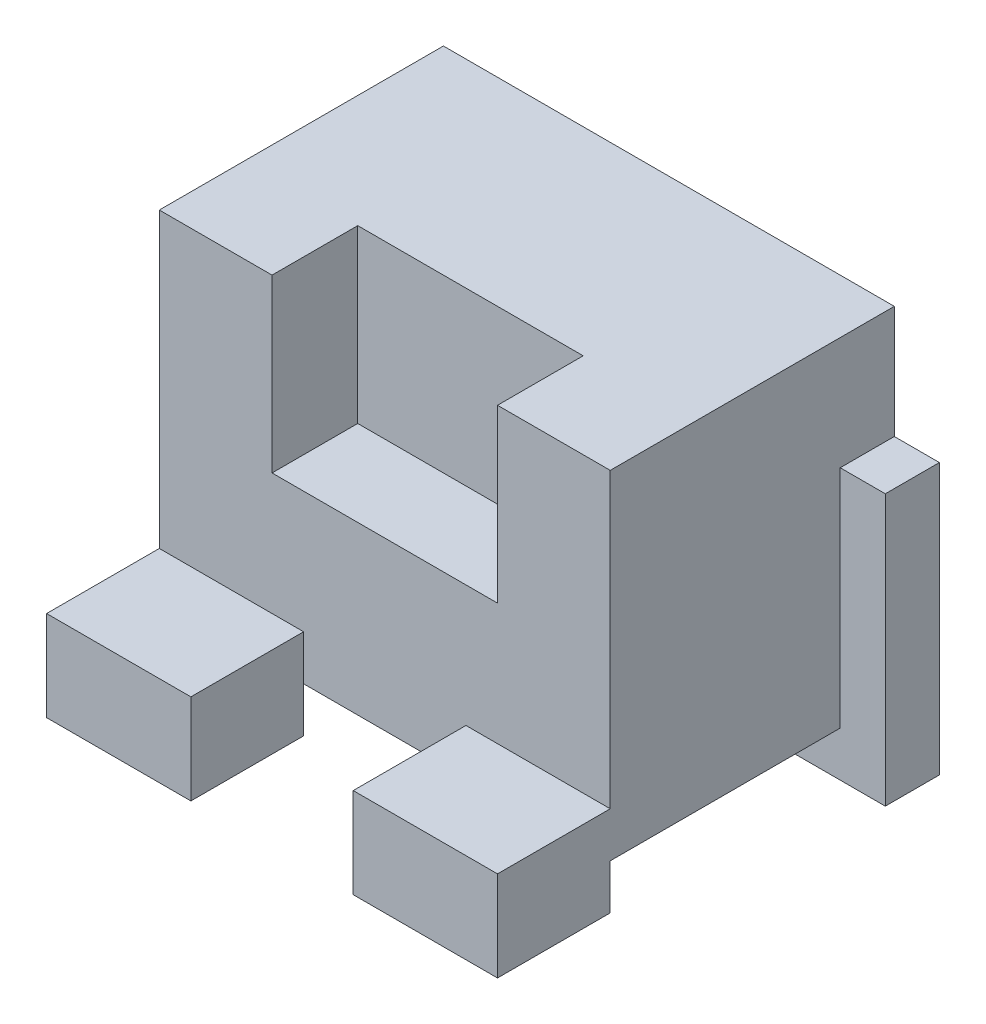
ISO-10303-21;
HEADER;
FILE_DESCRIPTION(('STEP AP214'),'2;1');
FILE_NAME('part.step','',(''),(''),'','','');
FILE_SCHEMA(('AUTOMOTIVE_DESIGN { 1 0 10303 214 1 1 1 1 }'));
ENDSEC;
DATA;
#1=APPLICATION_CONTEXT('core data for automotive mechanical design processes');
#2=APPLICATION_PROTOCOL_DEFINITION('international standard','automotive_design',2000,#1);
#3=PRODUCT_CONTEXT('',#1,'mechanical');
#4=PRODUCT('Part','Part','',(#3));
#5=PRODUCT_RELATED_PRODUCT_CATEGORY('part','',(#4));
#6=PRODUCT_DEFINITION_FORMATION('','',#4);
#7=PRODUCT_DEFINITION_CONTEXT('part definition',#1,'design');
#8=PRODUCT_DEFINITION('design','',#6,#7);
#9=PRODUCT_DEFINITION_SHAPE('','',#8);
#10=(LENGTH_UNIT() NAMED_UNIT(*) SI_UNIT(.MILLI.,.METRE.));
#11=(NAMED_UNIT(*) PLANE_ANGLE_UNIT() SI_UNIT($,.RADIAN.));
#12=(NAMED_UNIT(*) SI_UNIT($,.STERADIAN.) SOLID_ANGLE_UNIT());
#13=UNCERTAINTY_MEASURE_WITH_UNIT(LENGTH_MEASURE(1.E-05),#10,'distance_accuracy_value','');
#14=(GEOMETRIC_REPRESENTATION_CONTEXT(3) GLOBAL_UNCERTAINTY_ASSIGNED_CONTEXT((#13)) GLOBAL_UNIT_ASSIGNED_CONTEXT((#10,
#11,#12)) REPRESENTATION_CONTEXT('',''));
#15=CARTESIAN_POINT('',(0.,0.,0.));
#16=DIRECTION('',(0.,0.,1.));
#17=DIRECTION('',(1.,0.,0.));
#18=AXIS2_PLACEMENT_3D('',#15,#16,#17);
#19=CARTESIAN_POINT('',(100.,75.,-63.));
#20=DIRECTION('',(-1.,0.,0.));
#21=DIRECTION('',(0.,0.,1.));
#22=AXIS2_PLACEMENT_3D('',#19,#20,#21);
#23=PLANE('',#22);
#24=DIRECTION('',(0.,0.,1.));
#25=VECTOR('',#24,1.);
#26=CARTESIAN_POINT('',(100.,50.,-63.));
#27=LINE('',#26,#25);
#28=CARTESIAN_POINT('',(100.,50.,-63.));
#29=VERTEX_POINT('',#28);
#30=CARTESIAN_POINT('',(100.,50.,-51.));
#31=VERTEX_POINT('',#30);
#32=EDGE_CURVE('E231',#29,#31,#27,.T.);
#33=ORIENTED_EDGE('',*,*,#32,.F.);
#34=DIRECTION('',(0.,-1.,0.));
#35=VECTOR('',#34,1.);
#36=CARTESIAN_POINT('',(100.,75.,-63.));
#37=LINE('',#36,#35);
#38=CARTESIAN_POINT('',(100.,75.,-63.));
#39=VERTEX_POINT('',#38);
#40=EDGE_CURVE('E206',#39,#29,#37,.T.);
#41=ORIENTED_EDGE('',*,*,#40,.F.);
#42=DIRECTION('',(0.,0.,-1.));
#43=VECTOR('',#42,1.);
#44=CARTESIAN_POINT('',(100.,75.,-63.));
#45=LINE('',#44,#43);
#46=CARTESIAN_POINT('',(100.,75.,0.));
#47=VERTEX_POINT('',#46);
#48=EDGE_CURVE('E330',#47,#39,#45,.T.);
#49=ORIENTED_EDGE('',*,*,#48,.F.);
#50=DIRECTION('',(0.,-1.,0.));
#51=VECTOR('',#50,1.);
#52=CARTESIAN_POINT('',(100.,75.,0.));
#53=LINE('',#52,#51);
#54=CARTESIAN_POINT('',(100.,9.99999999999999,0.));
#55=VERTEX_POINT('',#54);
#56=EDGE_CURVE('E351',#47,#55,#53,.T.);
#57=ORIENTED_EDGE('',*,*,#56,.T.);
#58=DIRECTION('',(0.,0.,1.));
#59=VECTOR('',#58,1.);
#60=CARTESIAN_POINT('',(100.,10.,0.));
#61=LINE('',#60,#59);
#62=CARTESIAN_POINT('',(100.,10.,25.));
#63=VERTEX_POINT('',#62);
#64=EDGE_CURVE('E250',#55,#63,#61,.T.);
#65=ORIENTED_EDGE('',*,*,#64,.T.);
#66=DIRECTION('',(0.,1.,0.));
#67=VECTOR('',#66,1.);
#68=CARTESIAN_POINT('',(100.,-10.,25.));
#69=LINE('',#68,#67);
#70=CARTESIAN_POINT('',(100.,-10.,25.));
#71=VERTEX_POINT('',#70);
#72=EDGE_CURVE('E256',#71,#63,#69,.T.);
#73=ORIENTED_EDGE('',*,*,#72,.F.);
#74=DIRECTION('',(0.,0.,1.));
#75=VECTOR('',#74,1.);
#76=CARTESIAN_POINT('',(100.,-10.,0.));
#77=LINE('',#76,#75);
#78=CARTESIAN_POINT('',(100.,-10.,0.));
#79=VERTEX_POINT('',#78);
#80=EDGE_CURVE('E239',#79,#71,#77,.T.);
#81=ORIENTED_EDGE('',*,*,#80,.F.);
#82=DIRECTION('',(0.,1.,0.));
#83=VECTOR('',#82,1.);
#84=CARTESIAN_POINT('',(100.,-10.,0.));
#85=LINE('',#84,#83);
#86=CARTESIAN_POINT('',(100.,0.,0.));
#87=VERTEX_POINT('',#86);
#88=EDGE_CURVE('E261',#79,#87,#85,.T.);
#89=ORIENTED_EDGE('',*,*,#88,.T.);
#90=DIRECTION('',(0.,0.,-1.));
#91=VECTOR('',#90,1.);
#92=CARTESIAN_POINT('',(100.,0.,-63.));
#93=LINE('',#92,#91);
#94=CARTESIAN_POINT('',(100.,0.,-51.));
#95=VERTEX_POINT('',#94);
#96=EDGE_CURVE('E337',#87,#95,#93,.T.);
#97=ORIENTED_EDGE('',*,*,#96,.T.);
#98=DIRECTION('',(0.,-1.,0.));
#99=VECTOR('',#98,1.);
#100=CARTESIAN_POINT('',(100.,75.,-51.));
#101=LINE('',#100,#99);
#102=EDGE_CURVE('E207',#31,#95,#101,.T.);
#103=ORIENTED_EDGE('',*,*,#102,.F.);
#104=EDGE_LOOP('',(#33,#41,#49,#57,#65,#73,#81,#89,#97,#103));
#105=FACE_BOUND('',#104,.T.);
#106=ADVANCED_FACE('F39',(#105),#23,.F.);
#107=CARTESIAN_POINT('',(0.,0.,0.));
#108=DIRECTION('',(0.,-1.,0.));
#109=DIRECTION('',(0.,0.,-1.));
#110=AXIS2_PLACEMENT_3D('',#107,#108,#109);
#111=PLANE('',#110);
#112=DIRECTION('',(0.,0.,1.));
#113=VECTOR('',#112,1.);
#114=CARTESIAN_POINT('',(90.,0.,0.));
#115=LINE('',#114,#113);
#116=CARTESIAN_POINT('',(90.,0.,-63.));
#117=VERTEX_POINT('',#116);
#118=CARTESIAN_POINT('',(90.,0.,-51.));
#119=VERTEX_POINT('',#118);
#120=EDGE_CURVE('E50',#117,#119,#115,.T.);
#121=ORIENTED_EDGE('',*,*,#120,.T.);
#122=DIRECTION('',(1.,0.,0.));
#123=VECTOR('',#122,1.);
#124=CARTESIAN_POINT('',(0.,0.,-51.));
#125=LINE('',#124,#123);
#126=EDGE_CURVE('E11',#119,#95,#125,.T.);
#127=ORIENTED_EDGE('',*,*,#126,.T.);
#128=ORIENTED_EDGE('',*,*,#96,.F.);
#129=DIRECTION('',(1.,0.,0.));
#130=VECTOR('',#129,1.);
#131=CARTESIAN_POINT('',(100.,0.,0.));
#132=LINE('',#131,#130);
#133=CARTESIAN_POINT('',(68.,0.,0.));
#134=VERTEX_POINT('',#133);
#135=EDGE_CURVE('E318',#134,#87,#132,.T.);
#136=ORIENTED_EDGE('',*,*,#135,.F.);
#137=CARTESIAN_POINT('',(32.,0.,0.));
#138=VERTEX_POINT('',#137);
#139=EDGE_CURVE('E338',#138,#134,#132,.T.);
#140=ORIENTED_EDGE('',*,*,#139,.F.);
#141=CARTESIAN_POINT('',(0.,0.,0.));
#142=VERTEX_POINT('',#141);
#143=EDGE_CURVE('E333',#142,#138,#132,.T.);
#144=ORIENTED_EDGE('',*,*,#143,.F.);
#145=DIRECTION('',(0.,0.,1.));
#146=VECTOR('',#145,1.);
#147=CARTESIAN_POINT('',(0.,0.,0.));
#148=LINE('',#147,#146);
#149=CARTESIAN_POINT('',(0.,0.,-63.));
#150=VERTEX_POINT('',#149);
#151=EDGE_CURVE('E344',#150,#142,#148,.T.);
#152=ORIENTED_EDGE('',*,*,#151,.F.);
#153=DIRECTION('',(-1.,0.,0.));
#154=VECTOR('',#153,1.);
#155=CARTESIAN_POINT('',(0.,0.,-63.));
#156=LINE('',#155,#154);
#157=EDGE_CURVE('E345',#117,#150,#156,.T.);
#158=ORIENTED_EDGE('',*,*,#157,.F.);
#159=EDGE_LOOP('',(#121,#127,#128,#136,#140,#144,#152,#158));
#160=FACE_BOUND('',#159,.T.);
#161=ADVANCED_FACE('F383',(#160),#111,.T.);
#162=CARTESIAN_POINT('',(100.,75.,0.));
#163=DIRECTION('',(0.,0.,-1.));
#164=DIRECTION('',(-1.,0.,0.));
#165=AXIS2_PLACEMENT_3D('',#162,#163,#164);
#166=PLANE('',#165);
#167=DIRECTION('',(0.,1.,0.));
#168=VECTOR('',#167,1.);
#169=CARTESIAN_POINT('',(68.,-10.,0.));
#170=LINE('',#169,#168);
#171=CARTESIAN_POINT('',(68.,9.99999999999999,0.));
#172=VERTEX_POINT('',#171);
#173=EDGE_CURVE('E65',#134,#172,#170,.T.);
#174=ORIENTED_EDGE('',*,*,#173,.T.);
#175=DIRECTION('',(1.,0.,0.));
#176=VECTOR('',#175,1.);
#177=CARTESIAN_POINT('',(68.,10.,0.));
#178=LINE('',#177,#176);
#179=EDGE_CURVE('E232',#172,#55,#178,.T.);
#180=ORIENTED_EDGE('',*,*,#179,.T.);
#181=ORIENTED_EDGE('',*,*,#56,.F.);
#182=DIRECTION('',(1.,0.,0.));
#183=VECTOR('',#182,1.);
#184=CARTESIAN_POINT('',(100.,75.,0.));
#185=LINE('',#184,#183);
#186=CARTESIAN_POINT('',(75.,75.,0.));
#187=VERTEX_POINT('',#186);
#188=EDGE_CURVE('E327',#187,#47,#185,.T.);
#189=ORIENTED_EDGE('',*,*,#188,.F.);
#190=DIRECTION('',(0.,1.,0.));
#191=VECTOR('',#190,1.);
#192=CARTESIAN_POINT('',(75.,37.,0.));
#193=LINE('',#192,#191);
#194=CARTESIAN_POINT('',(75.,37.,0.));
#195=VERTEX_POINT('',#194);
#196=EDGE_CURVE('E299',#195,#187,#193,.T.);
#197=ORIENTED_EDGE('',*,*,#196,.F.);
#198=DIRECTION('',(1.,0.,0.));
#199=VECTOR('',#198,1.);
#200=CARTESIAN_POINT('',(25.,37.,0.));
#201=LINE('',#200,#199);
#202=CARTESIAN_POINT('',(25.,37.,0.));
#203=VERTEX_POINT('',#202);
#204=EDGE_CURVE('E313',#203,#195,#201,.T.);
#205=ORIENTED_EDGE('',*,*,#204,.F.);
#206=DIRECTION('',(0.,-1.,0.));
#207=VECTOR('',#206,1.);
#208=CARTESIAN_POINT('',(25.,75.,0.));
#209=LINE('',#208,#207);
#210=CARTESIAN_POINT('',(25.,75.,0.));
#211=VERTEX_POINT('',#210);
#212=EDGE_CURVE('E294',#211,#203,#209,.T.);
#213=ORIENTED_EDGE('',*,*,#212,.F.);
#214=CARTESIAN_POINT('',(0.,75.,0.));
#215=VERTEX_POINT('',#214);
#216=EDGE_CURVE('E322',#215,#211,#185,.T.);
#217=ORIENTED_EDGE('',*,*,#216,.F.);
#218=DIRECTION('',(0.,-1.,0.));
#219=VECTOR('',#218,1.);
#220=CARTESIAN_POINT('',(0.,75.,0.));
#221=LINE('',#220,#219);
#222=CARTESIAN_POINT('',(0.,9.99999999999999,0.));
#223=VERTEX_POINT('',#222);
#224=EDGE_CURVE('E331',#215,#223,#221,.T.);
#225=ORIENTED_EDGE('',*,*,#224,.T.);
#226=DIRECTION('',(1.,0.,0.));
#227=VECTOR('',#226,1.);
#228=CARTESIAN_POINT('',(32.,10.,0.));
#229=LINE('',#228,#227);
#230=CARTESIAN_POINT('',(32.,10.,0.));
#231=VERTEX_POINT('',#230);
#232=EDGE_CURVE('E262',#223,#231,#229,.T.);
#233=ORIENTED_EDGE('',*,*,#232,.T.);
#234=DIRECTION('',(0.,1.,0.));
#235=VECTOR('',#234,1.);
#236=CARTESIAN_POINT('',(32.,-10.,0.));
#237=LINE('',#236,#235);
#238=EDGE_CURVE('E293',#138,#231,#237,.T.);
#239=ORIENTED_EDGE('',*,*,#238,.F.);
#240=ORIENTED_EDGE('',*,*,#139,.T.);
#241=EDGE_LOOP('',(#174,#180,#181,#189,#197,#205,#213,#217,#225,#233,#239,#240));
#242=FACE_BOUND('',#241,.T.);
#243=ADVANCED_FACE('F41',(#242),#166,.F.);
#244=CARTESIAN_POINT('',(0.,75.,-63.));
#245=DIRECTION('',(0.,0.,1.));
#246=DIRECTION('',(1.,0.,0.));
#247=AXIS2_PLACEMENT_3D('',#244,#245,#246);
#248=PLANE('',#247);
#249=ORIENTED_EDGE('',*,*,#40,.T.);
#250=DIRECTION('',(-1.,0.,0.));
#251=VECTOR('',#250,1.);
#252=CARTESIAN_POINT('',(110.,50.,-63.));
#253=LINE('',#252,#251);
#254=CARTESIAN_POINT('',(110.,50.,-63.));
#255=VERTEX_POINT('',#254);
#256=EDGE_CURVE('E205',#255,#29,#253,.T.);
#257=ORIENTED_EDGE('',*,*,#256,.F.);
#258=DIRECTION('',(0.,1.,0.));
#259=VECTOR('',#258,1.);
#260=CARTESIAN_POINT('',(110.,-9.99999999999999,-63.));
#261=LINE('',#260,#259);
#262=CARTESIAN_POINT('',(110.,-9.99999999999999,-63.));
#263=VERTEX_POINT('',#262);
#264=EDGE_CURVE('E187',#263,#255,#261,.T.);
#265=ORIENTED_EDGE('',*,*,#264,.F.);
#266=DIRECTION('',(-1.,0.,0.));
#267=VECTOR('',#266,1.);
#268=CARTESIAN_POINT('',(110.,-9.99999999999999,-63.));
#269=LINE('',#268,#267);
#270=CARTESIAN_POINT('',(90.,-9.99999999999999,-63.));
#271=VERTEX_POINT('',#270);
#272=EDGE_CURVE('E219',#263,#271,#269,.T.);
#273=ORIENTED_EDGE('',*,*,#272,.T.);
#274=DIRECTION('',(0.,1.,0.));
#275=VECTOR('',#274,1.);
#276=CARTESIAN_POINT('',(90.,0.,-63.));
#277=LINE('',#276,#275);
#278=EDGE_CURVE('E222',#271,#117,#277,.T.);
#279=ORIENTED_EDGE('',*,*,#278,.T.);
#280=ORIENTED_EDGE('',*,*,#157,.T.);
#281=DIRECTION('',(0.,-1.,0.));
#282=VECTOR('',#281,1.);
#283=CARTESIAN_POINT('',(0.,75.,-63.));
#284=LINE('',#283,#282);
#285=CARTESIAN_POINT('',(0.,75.,-63.));
#286=VERTEX_POINT('',#285);
#287=EDGE_CURVE('E350',#286,#150,#284,.T.);
#288=ORIENTED_EDGE('',*,*,#287,.F.);
#289=DIRECTION('',(-1.,0.,0.));
#290=VECTOR('',#289,1.);
#291=CARTESIAN_POINT('',(0.,75.,-63.));
#292=LINE('',#291,#290);
#293=EDGE_CURVE('E329',#39,#286,#292,.T.);
#294=ORIENTED_EDGE('',*,*,#293,.F.);
#295=EDGE_LOOP('',(#249,#257,#265,#273,#279,#280,#288,#294));
#296=FACE_BOUND('',#295,.T.);
#297=ADVANCED_FACE('F201',(#296),#248,.F.);
#298=CARTESIAN_POINT('',(0.,75.,0.));
#299=DIRECTION('',(1.,0.,0.));
#300=DIRECTION('',(0.,0.,-1.));
#301=AXIS2_PLACEMENT_3D('',#298,#299,#300);
#302=PLANE('',#301);
#303=ORIENTED_EDGE('',*,*,#151,.T.);
#304=DIRECTION('',(0.,1.,0.));
#305=VECTOR('',#304,1.);
#306=CARTESIAN_POINT('',(0.,-10.,0.));
#307=LINE('',#306,#305);
#308=CARTESIAN_POINT('',(0.,-10.,0.));
#309=VERTEX_POINT('',#308);
#310=EDGE_CURVE('E274',#309,#142,#307,.T.);
#311=ORIENTED_EDGE('',*,*,#310,.F.);
#312=DIRECTION('',(0.,0.,-1.));
#313=VECTOR('',#312,1.);
#314=CARTESIAN_POINT('',(0.,-10.,0.));
#315=LINE('',#314,#313);
#316=CARTESIAN_POINT('',(0.,-10.,25.));
#317=VERTEX_POINT('',#316);
#318=EDGE_CURVE('E272',#317,#309,#315,.T.);
#319=ORIENTED_EDGE('',*,*,#318,.F.);
#320=DIRECTION('',(0.,1.,0.));
#321=VECTOR('',#320,1.);
#322=CARTESIAN_POINT('',(0.,-10.,25.));
#323=LINE('',#322,#321);
#324=CARTESIAN_POINT('',(0.,10.,25.));
#325=VERTEX_POINT('',#324);
#326=EDGE_CURVE('E284',#317,#325,#323,.T.);
#327=ORIENTED_EDGE('',*,*,#326,.T.);
#328=DIRECTION('',(0.,0.,-1.));
#329=VECTOR('',#328,1.);
#330=CARTESIAN_POINT('',(0.,10.,0.));
#331=LINE('',#330,#329);
#332=EDGE_CURVE('E267',#325,#223,#331,.T.);
#333=ORIENTED_EDGE('',*,*,#332,.T.);
#334=ORIENTED_EDGE('',*,*,#224,.F.);
#335=DIRECTION('',(0.,0.,1.));
#336=VECTOR('',#335,1.);
#337=CARTESIAN_POINT('',(0.,75.,0.));
#338=LINE('',#337,#336);
#339=EDGE_CURVE('E335',#286,#215,#338,.T.);
#340=ORIENTED_EDGE('',*,*,#339,.F.);
#341=ORIENTED_EDGE('',*,*,#287,.T.);
#342=EDGE_LOOP('',(#303,#311,#319,#327,#333,#334,#340,#341));
#343=FACE_BOUND('',#342,.T.);
#344=ADVANCED_FACE('F372',(#343),#302,.F.);
#345=CARTESIAN_POINT('',(0.,75.,0.));
#346=DIRECTION('',(0.,-1.,0.));
#347=DIRECTION('',(0.,0.,-1.));
#348=AXIS2_PLACEMENT_3D('',#345,#346,#347);
#349=PLANE('',#348);
#350=DIRECTION('',(-1.,0.,0.));
#351=VECTOR('',#350,1.);
#352=CARTESIAN_POINT('',(75.,75.,-19.));
#353=LINE('',#352,#351);
#354=CARTESIAN_POINT('',(75.,75.,-19.));
#355=VERTEX_POINT('',#354);
#356=CARTESIAN_POINT('',(25.,75.,-19.));
#357=VERTEX_POINT('',#356);
#358=EDGE_CURVE('E296',#355,#357,#353,.T.);
#359=ORIENTED_EDGE('',*,*,#358,.F.);
#360=DIRECTION('',(0.,0.,1.));
#361=VECTOR('',#360,1.);
#362=CARTESIAN_POINT('',(75.,75.,-19.));
#363=LINE('',#362,#361);
#364=EDGE_CURVE('E312',#355,#187,#363,.T.);
#365=ORIENTED_EDGE('',*,*,#364,.T.);
#366=ORIENTED_EDGE('',*,*,#188,.T.);
#367=ORIENTED_EDGE('',*,*,#48,.T.);
#368=ORIENTED_EDGE('',*,*,#293,.T.);
#369=ORIENTED_EDGE('',*,*,#339,.T.);
#370=ORIENTED_EDGE('',*,*,#216,.T.);
#371=DIRECTION('',(0.,0.,1.));
#372=VECTOR('',#371,1.);
#373=CARTESIAN_POINT('',(25.,75.,-19.));
#374=LINE('',#373,#372);
#375=EDGE_CURVE('E306',#357,#211,#374,.T.);
#376=ORIENTED_EDGE('',*,*,#375,.F.);
#377=EDGE_LOOP('',(#359,#365,#366,#367,#368,#369,#370,#376));
#378=FACE_BOUND('',#377,.T.);
#379=ADVANCED_FACE('F415',(#378),#349,.F.);
#380=CARTESIAN_POINT('',(75.,37.,-19.));
#381=DIRECTION('',(1.,0.,0.));
#382=DIRECTION('',(0.,0.,-1.));
#383=AXIS2_PLACEMENT_3D('',#380,#381,#382);
#384=PLANE('',#383);
#385=ORIENTED_EDGE('',*,*,#196,.T.);
#386=ORIENTED_EDGE('',*,*,#364,.F.);
#387=DIRECTION('',(0.,1.,0.));
#388=VECTOR('',#387,1.);
#389=CARTESIAN_POINT('',(75.,37.,-19.));
#390=LINE('',#389,#388);
#391=CARTESIAN_POINT('',(75.,37.,-19.));
#392=VERTEX_POINT('',#391);
#393=EDGE_CURVE('E308',#392,#355,#390,.T.);
#394=ORIENTED_EDGE('',*,*,#393,.F.);
#395=DIRECTION('',(0.,0.,1.));
#396=VECTOR('',#395,1.);
#397=CARTESIAN_POINT('',(75.,37.,-19.));
#398=LINE('',#397,#396);
#399=EDGE_CURVE('E317',#392,#195,#398,.T.);
#400=ORIENTED_EDGE('',*,*,#399,.T.);
#401=EDGE_LOOP('',(#385,#386,#394,#400));
#402=FACE_BOUND('',#401,.T.);
#403=ADVANCED_FACE('F420',(#402),#384,.F.);
#404=CARTESIAN_POINT('',(25.,37.,-19.));
#405=DIRECTION('',(0.,-1.,0.));
#406=DIRECTION('',(0.,0.,-1.));
#407=AXIS2_PLACEMENT_3D('',#404,#405,#406);
#408=PLANE('',#407);
#409=ORIENTED_EDGE('',*,*,#204,.T.);
#410=ORIENTED_EDGE('',*,*,#399,.F.);
#411=DIRECTION('',(1.,0.,0.));
#412=VECTOR('',#411,1.);
#413=CARTESIAN_POINT('',(25.,37.,-19.));
#414=LINE('',#413,#412);
#415=CARTESIAN_POINT('',(25.,37.,-19.));
#416=VERTEX_POINT('',#415);
#417=EDGE_CURVE('E301',#416,#392,#414,.T.);
#418=ORIENTED_EDGE('',*,*,#417,.F.);
#419=DIRECTION('',(0.,0.,1.));
#420=VECTOR('',#419,1.);
#421=CARTESIAN_POINT('',(25.,37.,-19.));
#422=LINE('',#421,#420);
#423=EDGE_CURVE('E321',#416,#203,#422,.T.);
#424=ORIENTED_EDGE('',*,*,#423,.T.);
#425=EDGE_LOOP('',(#409,#410,#418,#424));
#426=FACE_BOUND('',#425,.T.);
#427=ADVANCED_FACE('F421',(#426),#408,.F.);
#428=CARTESIAN_POINT('',(25.,75.,-19.));
#429=DIRECTION('',(-1.,0.,0.));
#430=DIRECTION('',(0.,0.,1.));
#431=AXIS2_PLACEMENT_3D('',#428,#429,#430);
#432=PLANE('',#431);
#433=ORIENTED_EDGE('',*,*,#212,.T.);
#434=ORIENTED_EDGE('',*,*,#423,.F.);
#435=DIRECTION('',(0.,-1.,0.));
#436=VECTOR('',#435,1.);
#437=CARTESIAN_POINT('',(25.,75.,-19.));
#438=LINE('',#437,#436);
#439=EDGE_CURVE('E298',#357,#416,#438,.T.);
#440=ORIENTED_EDGE('',*,*,#439,.F.);
#441=ORIENTED_EDGE('',*,*,#375,.T.);
#442=EDGE_LOOP('',(#433,#434,#440,#441));
#443=FACE_BOUND('',#442,.T.);
#444=ADVANCED_FACE('F422',(#443),#432,.F.);
#445=CARTESIAN_POINT('',(0.,0.,-19.));
#446=DIRECTION('',(0.,0.,1.));
#447=DIRECTION('',(1.,0.,0.));
#448=AXIS2_PLACEMENT_3D('',#445,#446,#447);
#449=PLANE('',#448);
#450=ORIENTED_EDGE('',*,*,#358,.T.);
#451=ORIENTED_EDGE('',*,*,#439,.T.);
#452=ORIENTED_EDGE('',*,*,#417,.T.);
#453=ORIENTED_EDGE('',*,*,#393,.T.);
#454=EDGE_LOOP('',(#450,#451,#452,#453));
#455=FACE_BOUND('',#454,.T.);
#456=ADVANCED_FACE('F456',(#455),#449,.T.);
#457=CARTESIAN_POINT('',(32.,-10.,0.));
#458=DIRECTION('',(0.,0.,1.));
#459=DIRECTION('',(1.,0.,0.));
#460=AXIS2_PLACEMENT_3D('',#457,#458,#459);
#461=PLANE('',#460);
#462=ORIENTED_EDGE('',*,*,#310,.T.);
#463=ORIENTED_EDGE('',*,*,#143,.T.);
#464=CARTESIAN_POINT('',(32.,-10.,0.));
#465=VERTEX_POINT('',#464);
#466=EDGE_CURVE('E292',#465,#138,#237,.T.);
#467=ORIENTED_EDGE('',*,*,#466,.F.);
#468=DIRECTION('',(1.,0.,0.));
#469=VECTOR('',#468,1.);
#470=CARTESIAN_POINT('',(32.,-10.,0.));
#471=LINE('',#470,#469);
#472=EDGE_CURVE('E264',#309,#465,#471,.T.);
#473=ORIENTED_EDGE('',*,*,#472,.F.);
#474=EDGE_LOOP('',(#462,#463,#467,#473));
#475=FACE_BOUND('',#474,.T.);
#476=ADVANCED_FACE('F381',(#475),#461,.F.);
#477=CARTESIAN_POINT('',(32.,-10.,25.));
#478=DIRECTION('',(-1.,0.,0.));
#479=DIRECTION('',(0.,0.,1.));
#480=AXIS2_PLACEMENT_3D('',#477,#478,#479);
#481=PLANE('',#480);
#482=DIRECTION('',(0.,0.,1.));
#483=VECTOR('',#482,1.);
#484=CARTESIAN_POINT('',(32.,10.,25.));
#485=LINE('',#484,#483);
#486=CARTESIAN_POINT('',(32.,10.,25.));
#487=VERTEX_POINT('',#486);
#488=EDGE_CURVE('E280',#231,#487,#485,.T.);
#489=ORIENTED_EDGE('',*,*,#488,.T.);
#490=DIRECTION('',(0.,1.,0.));
#491=VECTOR('',#490,1.);
#492=CARTESIAN_POINT('',(32.,-10.,25.));
#493=LINE('',#492,#491);
#494=CARTESIAN_POINT('',(32.,-10.,25.));
#495=VERTEX_POINT('',#494);
#496=EDGE_CURVE('E286',#495,#487,#493,.T.);
#497=ORIENTED_EDGE('',*,*,#496,.F.);
#498=DIRECTION('',(0.,0.,1.));
#499=VECTOR('',#498,1.);
#500=CARTESIAN_POINT('',(32.,-10.,25.));
#501=LINE('',#500,#499);
#502=EDGE_CURVE('E268',#465,#495,#501,.T.);
#503=ORIENTED_EDGE('',*,*,#502,.F.);
#504=ORIENTED_EDGE('',*,*,#466,.T.);
#505=ORIENTED_EDGE('',*,*,#238,.T.);
#506=EDGE_LOOP('',(#489,#497,#503,#504,#505));
#507=FACE_BOUND('',#506,.T.);
#508=ADVANCED_FACE('F359',(#507),#481,.F.);
#509=CARTESIAN_POINT('',(0.,-10.,25.));
#510=DIRECTION('',(0.,0.,-1.));
#511=DIRECTION('',(-1.,0.,0.));
#512=AXIS2_PLACEMENT_3D('',#509,#510,#511);
#513=PLANE('',#512);
#514=DIRECTION('',(-1.,0.,0.));
#515=VECTOR('',#514,1.);
#516=CARTESIAN_POINT('',(0.,10.,25.));
#517=LINE('',#516,#515);
#518=EDGE_CURVE('E276',#487,#325,#517,.T.);
#519=ORIENTED_EDGE('',*,*,#518,.T.);
#520=ORIENTED_EDGE('',*,*,#326,.F.);
#521=DIRECTION('',(-1.,0.,0.));
#522=VECTOR('',#521,1.);
#523=CARTESIAN_POINT('',(0.,-10.,25.));
#524=LINE('',#523,#522);
#525=EDGE_CURVE('E271',#495,#317,#524,.T.);
#526=ORIENTED_EDGE('',*,*,#525,.F.);
#527=ORIENTED_EDGE('',*,*,#496,.T.);
#528=EDGE_LOOP('',(#519,#520,#526,#527));
#529=FACE_BOUND('',#528,.T.);
#530=ADVANCED_FACE('F367',(#529),#513,.F.);
#531=CARTESIAN_POINT('',(0.,-10.,0.));
#532=DIRECTION('',(0.,1.,0.));
#533=DIRECTION('',(0.,0.,1.));
#534=AXIS2_PLACEMENT_3D('',#531,#532,#533);
#535=PLANE('',#534);
#536=ORIENTED_EDGE('',*,*,#472,.T.);
#537=ORIENTED_EDGE('',*,*,#502,.T.);
#538=ORIENTED_EDGE('',*,*,#525,.T.);
#539=ORIENTED_EDGE('',*,*,#318,.T.);
#540=EDGE_LOOP('',(#536,#537,#538,#539));
#541=FACE_BOUND('',#540,.T.);
#542=ADVANCED_FACE('F377',(#541),#535,.F.);
#543=CARTESIAN_POINT('',(0.,10.,0.));
#544=DIRECTION('',(0.,1.,0.));
#545=DIRECTION('',(0.,0.,1.));
#546=AXIS2_PLACEMENT_3D('',#543,#544,#545);
#547=PLANE('',#546);
#548=ORIENTED_EDGE('',*,*,#232,.F.);
#549=ORIENTED_EDGE('',*,*,#332,.F.);
#550=ORIENTED_EDGE('',*,*,#518,.F.);
#551=ORIENTED_EDGE('',*,*,#488,.F.);
#552=EDGE_LOOP('',(#548,#549,#550,#551));
#553=FACE_BOUND('',#552,.T.);
#554=ADVANCED_FACE('F368',(#553),#547,.T.);
#555=CARTESIAN_POINT('',(68.,-10.,0.));
#556=DIRECTION('',(0.,0.,1.));
#557=DIRECTION('',(1.,0.,0.));
#558=AXIS2_PLACEMENT_3D('',#555,#556,#557);
#559=PLANE('',#558);
#560=ORIENTED_EDGE('',*,*,#135,.T.);
#561=ORIENTED_EDGE('',*,*,#88,.F.);
#562=DIRECTION('',(1.,0.,0.));
#563=VECTOR('',#562,1.);
#564=CARTESIAN_POINT('',(68.,-10.,0.));
#565=LINE('',#564,#563);
#566=CARTESIAN_POINT('',(68.,-10.,0.));
#567=VERTEX_POINT('',#566);
#568=EDGE_CURVE('E237',#567,#79,#565,.T.);
#569=ORIENTED_EDGE('',*,*,#568,.F.);
#570=EDGE_CURVE('E252',#567,#134,#170,.T.);
#571=ORIENTED_EDGE('',*,*,#570,.T.);
#572=EDGE_LOOP('',(#560,#561,#569,#571));
#573=FACE_BOUND('',#572,.T.);
#574=ADVANCED_FACE('F389',(#573),#559,.F.);
#575=CARTESIAN_POINT('',(100.,-10.,25.));
#576=DIRECTION('',(0.,0.,-1.));
#577=DIRECTION('',(-1.,0.,0.));
#578=AXIS2_PLACEMENT_3D('',#575,#576,#577);
#579=PLANE('',#578);
#580=DIRECTION('',(-1.,0.,0.));
#581=VECTOR('',#580,1.);
#582=CARTESIAN_POINT('',(100.,10.,25.));
#583=LINE('',#582,#581);
#584=CARTESIAN_POINT('',(68.,10.,25.));
#585=VERTEX_POINT('',#584);
#586=EDGE_CURVE('E249',#63,#585,#583,.T.);
#587=ORIENTED_EDGE('',*,*,#586,.T.);
#588=DIRECTION('',(0.,1.,0.));
#589=VECTOR('',#588,1.);
#590=CARTESIAN_POINT('',(68.,-10.,25.));
#591=LINE('',#590,#589);
#592=CARTESIAN_POINT('',(68.,-10.,25.));
#593=VERTEX_POINT('',#592);
#594=EDGE_CURVE('E254',#593,#585,#591,.T.);
#595=ORIENTED_EDGE('',*,*,#594,.F.);
#596=DIRECTION('',(-1.,0.,0.));
#597=VECTOR('',#596,1.);
#598=CARTESIAN_POINT('',(100.,-10.,25.));
#599=LINE('',#598,#597);
#600=EDGE_CURVE('E245',#71,#593,#599,.T.);
#601=ORIENTED_EDGE('',*,*,#600,.F.);
#602=ORIENTED_EDGE('',*,*,#72,.T.);
#603=EDGE_LOOP('',(#587,#595,#601,#602));
#604=FACE_BOUND('',#603,.T.);
#605=ADVANCED_FACE('F476',(#604),#579,.F.);
#606=CARTESIAN_POINT('',(68.,-10.,25.));
#607=DIRECTION('',(1.,0.,0.));
#608=DIRECTION('',(0.,0.,-1.));
#609=AXIS2_PLACEMENT_3D('',#606,#607,#608);
#610=PLANE('',#609);
#611=DIRECTION('',(0.,0.,-1.));
#612=VECTOR('',#611,1.);
#613=CARTESIAN_POINT('',(68.,10.,25.));
#614=LINE('',#613,#612);
#615=EDGE_CURVE('E238',#585,#172,#614,.T.);
#616=ORIENTED_EDGE('',*,*,#615,.T.);
#617=ORIENTED_EDGE('',*,*,#173,.F.);
#618=ORIENTED_EDGE('',*,*,#570,.F.);
#619=DIRECTION('',(0.,0.,-1.));
#620=VECTOR('',#619,1.);
#621=CARTESIAN_POINT('',(68.,-10.,25.));
#622=LINE('',#621,#620);
#623=EDGE_CURVE('E243',#593,#567,#622,.T.);
#624=ORIENTED_EDGE('',*,*,#623,.F.);
#625=ORIENTED_EDGE('',*,*,#594,.T.);
#626=EDGE_LOOP('',(#616,#617,#618,#624,#625));
#627=FACE_BOUND('',#626,.T.);
#628=ADVANCED_FACE('F397',(#627),#610,.F.);
#629=CARTESIAN_POINT('',(0.,-10.,0.));
#630=DIRECTION('',(0.,-1.,0.));
#631=DIRECTION('',(0.,0.,-1.));
#632=AXIS2_PLACEMENT_3D('',#629,#630,#631);
#633=PLANE('',#632);
#634=ORIENTED_EDGE('',*,*,#568,.T.);
#635=ORIENTED_EDGE('',*,*,#80,.T.);
#636=ORIENTED_EDGE('',*,*,#600,.T.);
#637=ORIENTED_EDGE('',*,*,#623,.T.);
#638=EDGE_LOOP('',(#634,#635,#636,#637));
#639=FACE_BOUND('',#638,.T.);
#640=ADVANCED_FACE('F398',(#639),#633,.T.);
#641=CARTESIAN_POINT('',(0.,10.,0.));
#642=DIRECTION('',(0.,-1.,0.));
#643=DIRECTION('',(0.,0.,-1.));
#644=AXIS2_PLACEMENT_3D('',#641,#642,#643);
#645=PLANE('',#644);
#646=ORIENTED_EDGE('',*,*,#179,.F.);
#647=ORIENTED_EDGE('',*,*,#615,.F.);
#648=ORIENTED_EDGE('',*,*,#586,.F.);
#649=ORIENTED_EDGE('',*,*,#64,.F.);
#650=EDGE_LOOP('',(#646,#647,#648,#649));
#651=FACE_BOUND('',#650,.T.);
#652=ADVANCED_FACE('F406',(#651),#645,.F.);
#653=CARTESIAN_POINT('',(110.,50.,-63.));
#654=DIRECTION('',(0.,-1.,0.));
#655=DIRECTION('',(0.,0.,-1.));
#656=AXIS2_PLACEMENT_3D('',#653,#654,#655);
#657=PLANE('',#656);
#658=ORIENTED_EDGE('',*,*,#256,.T.);
#659=ORIENTED_EDGE('',*,*,#32,.T.);
#660=DIRECTION('',(-1.,0.,0.));
#661=VECTOR('',#660,1.);
#662=CARTESIAN_POINT('',(110.,50.,-51.));
#663=LINE('',#662,#661);
#664=CARTESIAN_POINT('',(110.,50.,-51.));
#665=VERTEX_POINT('',#664);
#666=EDGE_CURVE('E209',#665,#31,#663,.T.);
#667=ORIENTED_EDGE('',*,*,#666,.F.);
#668=DIRECTION('',(0.,0.,1.));
#669=VECTOR('',#668,1.);
#670=CARTESIAN_POINT('',(110.,50.,-63.));
#671=LINE('',#670,#669);
#672=EDGE_CURVE('E195',#255,#665,#671,.T.);
#673=ORIENTED_EDGE('',*,*,#672,.F.);
#674=EDGE_LOOP('',(#658,#659,#667,#673));
#675=FACE_BOUND('',#674,.T.);
#676=ADVANCED_FACE('F215',(#675),#657,.F.);
#677=CARTESIAN_POINT('',(110.,50.,-51.));
#678=DIRECTION('',(0.,0.,-1.));
#679=DIRECTION('',(0.,1.,0.));
#680=AXIS2_PLACEMENT_3D('',#677,#678,#679);
#681=PLANE('',#680);
#682=ORIENTED_EDGE('',*,*,#666,.T.);
#683=ORIENTED_EDGE('',*,*,#102,.T.);
#684=ORIENTED_EDGE('',*,*,#126,.F.);
#685=DIRECTION('',(0.,-1.,0.));
#686=VECTOR('',#685,1.);
#687=CARTESIAN_POINT('',(90.,50.,-51.));
#688=LINE('',#687,#686);
#689=CARTESIAN_POINT('',(90.,-9.99999999999999,-51.));
#690=VERTEX_POINT('',#689);
#691=EDGE_CURVE('E53',#119,#690,#688,.T.);
#692=ORIENTED_EDGE('',*,*,#691,.T.);
#693=DIRECTION('',(-1.,0.,0.));
#694=VECTOR('',#693,1.);
#695=CARTESIAN_POINT('',(110.,-9.99999999999999,-51.));
#696=LINE('',#695,#694);
#697=CARTESIAN_POINT('',(110.,-9.99999999999999,-51.));
#698=VERTEX_POINT('',#697);
#699=EDGE_CURVE('E227',#698,#690,#696,.T.);
#700=ORIENTED_EDGE('',*,*,#699,.F.);
#701=DIRECTION('',(0.,-1.,0.));
#702=VECTOR('',#701,1.);
#703=CARTESIAN_POINT('',(110.,50.,-51.));
#704=LINE('',#703,#702);
#705=EDGE_CURVE('E214',#665,#698,#704,.T.);
#706=ORIENTED_EDGE('',*,*,#705,.F.);
#707=EDGE_LOOP('',(#682,#683,#684,#692,#700,#706));
#708=FACE_BOUND('',#707,.T.);
#709=ADVANCED_FACE('F432',(#708),#681,.F.);
#710=CARTESIAN_POINT('',(110.,-9.99999999999999,-51.));
#711=DIRECTION('',(0.,1.,0.));
#712=DIRECTION('',(0.,0.,1.));
#713=AXIS2_PLACEMENT_3D('',#710,#711,#712);
#714=PLANE('',#713);
#715=DIRECTION('',(0.,0.,-1.));
#716=VECTOR('',#715,1.);
#717=CARTESIAN_POINT('',(90.,-9.99999999999999,-51.));
#718=LINE('',#717,#716);
#719=EDGE_CURVE('E200',#690,#271,#718,.T.);
#720=ORIENTED_EDGE('',*,*,#719,.T.);
#721=ORIENTED_EDGE('',*,*,#272,.F.);
#722=DIRECTION('',(0.,0.,-1.));
#723=VECTOR('',#722,1.);
#724=CARTESIAN_POINT('',(110.,-9.99999999999999,-51.));
#725=LINE('',#724,#723);
#726=EDGE_CURVE('E192',#698,#263,#725,.T.);
#727=ORIENTED_EDGE('',*,*,#726,.F.);
#728=ORIENTED_EDGE('',*,*,#699,.T.);
#729=EDGE_LOOP('',(#720,#721,#727,#728));
#730=FACE_BOUND('',#729,.T.);
#731=ADVANCED_FACE('F431',(#730),#714,.F.);
#732=CARTESIAN_POINT('',(110.,0.,0.));
#733=DIRECTION('',(1.,0.,0.));
#734=DIRECTION('',(0.,0.,-1.));
#735=AXIS2_PLACEMENT_3D('',#732,#733,#734);
#736=PLANE('',#735);
#737=ORIENTED_EDGE('',*,*,#264,.T.);
#738=ORIENTED_EDGE('',*,*,#672,.T.);
#739=ORIENTED_EDGE('',*,*,#705,.T.);
#740=ORIENTED_EDGE('',*,*,#726,.T.);
#741=EDGE_LOOP('',(#737,#738,#739,#740));
#742=FACE_BOUND('',#741,.T.);
#743=ADVANCED_FACE('F189',(#742),#736,.T.);
#744=CARTESIAN_POINT('',(90.,0.,0.));
#745=DIRECTION('',(1.,0.,0.));
#746=DIRECTION('',(0.,0.,-1.));
#747=AXIS2_PLACEMENT_3D('',#744,#745,#746);
#748=PLANE('',#747);
#749=ORIENTED_EDGE('',*,*,#120,.F.);
#750=ORIENTED_EDGE('',*,*,#278,.F.);
#751=ORIENTED_EDGE('',*,*,#719,.F.);
#752=ORIENTED_EDGE('',*,*,#691,.F.);
#753=EDGE_LOOP('',(#749,#750,#751,#752));
#754=FACE_BOUND('',#753,.T.);
#755=ADVANCED_FACE('F427',(#754),#748,.F.);
#756=CLOSED_SHELL('',(#106,#161,#243,#297,#344,#379,#403,#427,#444,#456,#476,#508,#530,#542,
#554,#574,#605,#628,#640,#652,#676,#709,#731,#743,#755));
#757=MANIFOLD_SOLID_BREP('B2',#756);
#758=ADVANCED_BREP_SHAPE_REPRESENTATION('',(#18,#757),#14);
#759=SHAPE_DEFINITION_REPRESENTATION(#9,#758);
ENDSEC;
END-ISO-10303-21;
